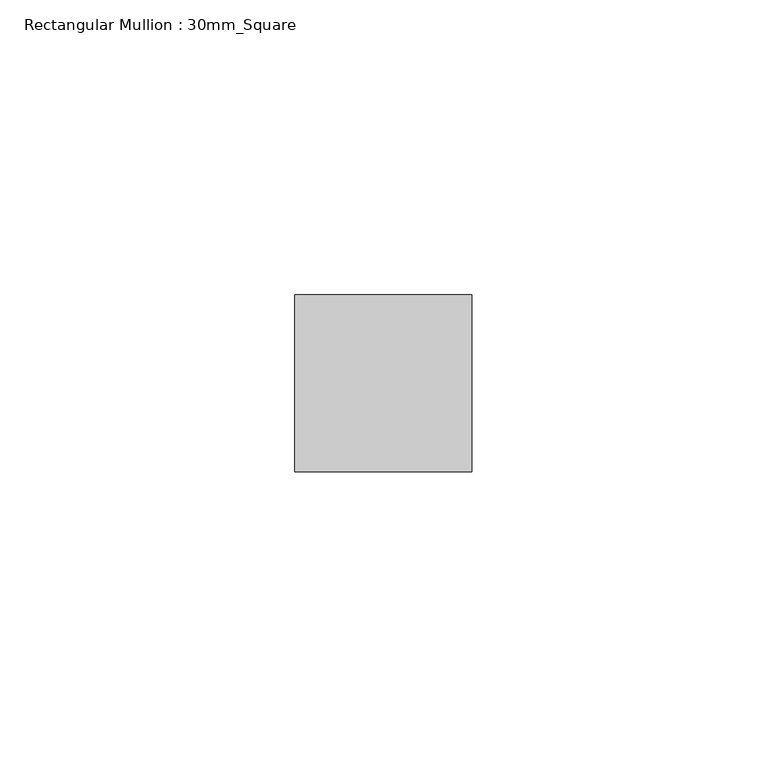
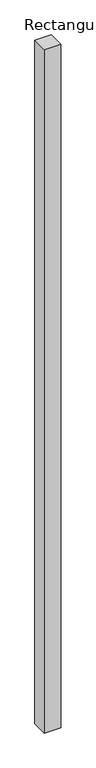
"""IFC4 building model written with IfcOpenShell, lengths in millimetres: member geometry, Rectangular Mullion : 30mm_Square."""

from ifc_helpers import new_model, si_unit, frame, origin, place, context, project, spatial, polyline, outline, extrude, source, transform, mapped, element, save


def rectangular_mullion_30mm_square_7ad516a4(model_context):
    return source(origin(), model_context, "Body", "SweptSolid", [
        extrude(outline(polyline([(15.0, 15.0), (15.0, -15.0), (-15.0, -15.0), (-15.0, 15.0), (15.0, 15.0)])), frame((0.0, 0.0, -1330.8429687), z_axis=(0.0, 0.0, 1.0), x_axis=(1.0, 0.0, 0.0)), (0.0, 0.0, 1.0), 1330.8429687),
    ])


if __name__ == "__main__":
    model = new_model("IFC4")
    model_context = context("Model", 3, world=origin())
    ifc_project = project(units=[si_unit("LENGTHUNIT", "METRE", prefix="MILLI")], contexts=[model_context])
    site = spatial("IfcSite", under=ifc_project)
    building = spatial("IfcBuilding", under=site)
    placement = place(None, origin())
    rectangular_mullion_30mm_square_shape = rectangular_mullion_30mm_square_7ad516a4(model_context)
    element("IfcMember", 1, ObjectType="Rectangular Mullion : 30mm_Square", at=placement, inside=building, context=model_context, shape_type="MappedRepresentation", body=[
        mapped(rectangular_mullion_30mm_square_shape, transform((0.0, 0.0, 0.0), x_axis=(1.0, 0.0, 0.0), y_axis=(0.0, 1.0, 0.0), z_axis=(0.0, 0.0, 1.0))),
    ])
    save(model, "model.ifc")

# Revit data of these elements
# Type "Rectangular Mullion : 30mm_Square"
#   Keynote = "H11"
#   built-in parameter 1007304 = 0.0984252 (stored number, unit not read)
#   built-in parameter 1007301 = 0.0492126 (stored number, unit not read)
#   built-in parameter 1007300 = 0.0492126 (stored number, unit not read)
# Element 1 (IfcMember, "Rectangular Mullion : 30mm_Square")
#   Materials on its faces: "Aluminium"
# Materials
#   "Aluminium": class "Metal", colour RGB 247 247 247, transparency 0, Description = "Aluminium 6061", Cost = 0
